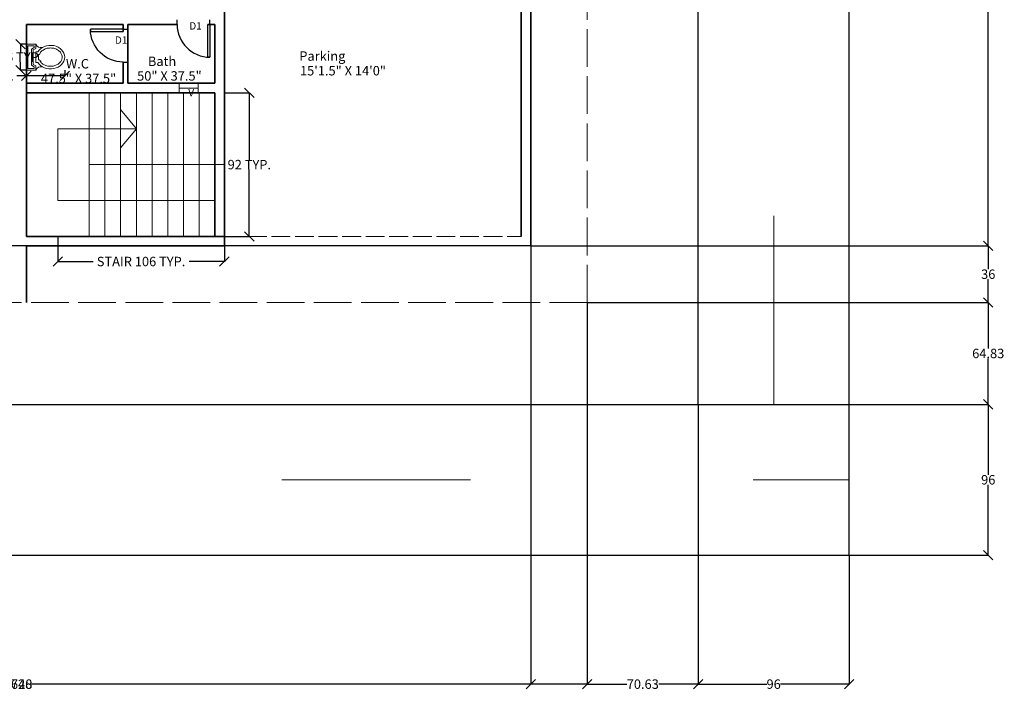
# Model space of a CAD drawing. Units: inches. Extents: x -1198 to -69, y -512 to 437.
# Tile 26 of 50: x -696 to -69, y -512 to -85. Entities that reach past the tile are written whole.
import ezdxf

# ---------------------------------------------------------------- set-up
doc = ezdxf.new("R2010")
doc.units = ezdxf.units.IN
doc.header["$MEASUREMENT"] = 0
doc.linetypes.add('ACAD_ISO02W100', pattern=[15, 12, -3])
doc.linetypes.add('ACAD_ISO03W100', pattern=[30, 12, -18])
for name, color, linetype, lineweight in [('A-ANNO-DIMS', 2, 'Continuous', 18), ('A-ANNO-SYMB', 7, 'Continuous', 18), ('A-AREA-IDEN', 7, 'Continuous', 18), ('A-FLOR-FIXT', 60, 'Continuous', 18), ('A-FLOR-OPEN', 7, 'ACAD_ISO02W100', 18), ('A-FLOR-STRS', 7, 'Continuous', 18), ('A-WALL', 7, 'Continuous', 35), ('C-PROP', 141, 'ACAD_ISO02W100', 18), ('C-ROAD', 7, 'Continuous', 25), ('C-ROAD-CNTR', 7, 'ACAD_ISO03W100', 18), ('Doors', 140, 'Continuous', 25), ('windows', 160, 'Continuous', 18)]:
    doc.layers.add(name, color=color, linetype=linetype, lineweight=lineweight)
doc.styles.get("Standard").update_dxf_attribs({"font": 'arial.ttf'})
doc.dimstyles.get("Standard").update_dxf_attribs({"dimtxt": 6, "dimasz": 6, "dimexe": 0.18, "dimexo": 0.0625, "dimgap": 0.09, "dimtad": 0, "dimtih": 1, "dimtoh": 1, "dimdec": 0, "dimzin": 0, "dimdsep": 46, "dimlunit": 4, "dimtxsty": 'Standard', "dimblk": 'OBLIQUE', "dimcen": 0.09, "dimadec": 0, "dimazin": 0, "dimtfac": 1, "dimtdec": 0, "dimtofl": 0, "dimtmove": 0, "dimatfit": 3, "dimfxl": 1, "dimtolj": 1, "dimtzin": 0, "dimarcsym": 0})

# ---------------------------------------------------------------- blocks, each defined once
blk = doc.blocks.new('A$C7C8779AE')
for p, q in [((0, 0.74), (0, 0.56)), ((0.5, 0.74), (0, 0.74)), ((0.47, 0.71), (0.03, 0.71)), ((0.03, 0.71), (0.03, 0.59)), ((0.03, 0.59), (0.063, 0.59)), ((0.093, 0.64), (0.063, 0.59)), ((0.11, 0.61), (0.08, 0.56)), ((0.093, 0.64), (0.407, 0.64)), ((0.11, 0.61), (0.39, 0.61)), ((0.42, 0.56), (0.39, 0.61)), ((0.437, 0.59), (0.407, 0.64)), ((0.437, 0.59), (0.47, 0.59)), ((0.47, 0.59), (0.47, 0.71)), ((0.5, 0.56), (0.5, 0.74)), ((0, 0.56), (0.08, 0.56)), ((0.15, 0.557), (0.15, 0.52)), ((0.15, 0.557), (0.351, 0.557)), ((0.2, 0.507), (0.2, 0.488)), ((0.2, 0.507), (0.301, 0.507)), ((0.301, 0.507), (0.301, 0.488)), ((0.351, 0.557), (0.351, 0.52)), ((0.42, 0.56), (0.5, 0.56))]:
    blk.add_line(p, q)
for centre, start, end in [((-0.039, 0.461), 344.642, 68.7339), ((0.539, 0.461), 111.2661, 195.358)]:
    blk.add_arc(centre, 0.106, start, end)
blk.add_ellipse((0.251, 0.274), major_axis=(0, 0.274), ratio=0.828948, start_param=0.459479, end_param=5.823706)
blk.add_open_spline([(0.2, 0.488), (0.17, 0.474), (0.164, 0.47), (0.151, 0.46), (0.144, 0.454), (0.13, 0.439), (0.123, 0.431), (0.111, 0.413), (0.106, 0.404), (0.096, 0.384), (0.091, 0.373), (0.084, 0.352), (0.081, 0.34), (0.076, 0.317), (0.075, 0.305), (0.073, 0.282), (0.073, 0.27), (0.074, 0.246), (0.076, 0.234), (0.08, 0.211), (0.083, 0.2), (0.09, 0.178), (0.095, 0.167), (0.104, 0.147), (0.11, 0.138), (0.122, 0.12), (0.128, 0.112), (0.142, 0.097), (0.149, 0.09), (0.165, 0.078), (0.173, 0.073), (0.189, 0.064), (0.197, 0.06), (0.214, 0.055), (0.222, 0.053), (0.239, 0.05), (0.248, 0.05), (0.266, 0.051), (0.276, 0.052), (0.296, 0.057), (0.306, 0.061), (0.325, 0.071), (0.335, 0.077), (0.353, 0.091), (0.361, 0.099), (0.377, 0.117), (0.384, 0.127), (0.398, 0.149), (0.404, 0.161), (0.414, 0.185), (0.418, 0.198), (0.424, 0.225), (0.426, 0.239), (0.428, 0.267), (0.428, 0.281), (0.426, 0.309), (0.424, 0.323), (0.418, 0.349), (0.414, 0.363), (0.404, 0.387), (0.398, 0.399), (0.385, 0.421), (0.378, 0.431), (0.362, 0.449), (0.353, 0.458), (0.338, 0.469), (0.332, 0.474), (0.301, 0.488)], degree=3, knots=[0.459479, 0.459479, 0.459479, 0.459479, 0.567422, 0.567422, 0.720865, 0.720865, 0.874307, 0.874307, 1.02775, 1.02775, 1.181192, 1.181192, 1.334635, 1.334635, 1.488077, 1.488077, 1.64152, 1.64152, 1.794963, 1.794963, 1.948405, 1.948405, 2.101848, 2.101848, 2.25529, 2.25529, 2.408733, 2.408733, 2.562175, 2.562175, 2.715618, 2.715618, 2.86906, 2.86906, 3.022503, 3.022503, 3.175946, 3.175946, 3.356457, 3.356457, 3.536968, 3.536968, 3.717479, 3.717479, 3.89799, 3.89799, 4.078501, 4.078501, 4.259012, 4.259012, 4.439523, 4.439523, 4.620035, 4.620035, 4.800546, 4.800546, 4.981057, 4.981057, 5.161568, 5.161568, 5.342079, 5.342079, 5.52259, 5.52259, 5.703101, 5.703101, 5.823706, 5.823706, 5.823706, 5.823706])
blk = doc.blocks.new('A')
at = {"xscale": 1000, "yscale": 1000, "zscale": 1000}
blk.add_blockref('A$C7C8779AE', (-251, 0), dxfattribs=at)
blk = doc.blocks.new('VENT-12')
at = {"ltscale": 10}
for p, q in [((0, 6), (0, 0)), ((0, 3), (12, 3)), ((12, 6), (12, 0))]:
    blk.add_line(p, q, dxfattribs=at)
blk = doc.blocks.new('DOOR-D1-JAMB3')
for p, q in [((0, 0), (0, -3)), ((20.87, 0), (20.87, -3))]:
    blk.add_line(p, q)
blk.add_lwpolyline([(0, 0), (0, 20.87), (1.3, 20.87), (1.3, 0)], close=True)
blk.add_arc((0, 0), 20.87, 0, 90)
blk = doc.blocks.new('STAIR-RETURN')
at = {"ltscale": 10}
for p, q in [((20, 91.5), (20, 0)), ((30, 91.5), (30, 0)), ((40, 91.5), (40, 0)), ((50, 91.5), (50, 0)), ((60, 91.5), (60, 0)), ((70, 91.5), (70, 0)), ((80, 91.5), (80, 0)), ((90, 91.5), (90, 0)), ((50, 68.62), (40, 80.86)), ((0, 22.87), (0, 68.62)), ((0, 68.62), (50, 68.62)), ((50, 68.62), (40, 56.39)), ((20, 45.75), (106, 45.75)), ((100, 22.87), (0, 22.87))]:
    blk.add_line(p, q, dxfattribs=at)
blk = doc.blocks.new('_Oblique')
at = {"color": 0, "linetype": 'ByBlock', "lineweight": -2}
blk.add_line((-0.5, -0.5), (0.5, 0.5), dxfattribs=at)
blk = doc.blocks.new('*D44')
at = {"layer": 'A-ANNO-DIMS', "color": 0, "lineweight": -2, "ltscale": 10, "transparency": 16777216}
for p, q in [((-691.75, -116.92), (-691.75, -120.7)), ((-667.34, -116.92), (-667.34, -120.7)), ((-691.75, -120.52), (-697.75, -120.52)), ((-667.34, -120.52), (-691.75, -120.52))]:
    blk.add_line(p, q, dxfattribs=at)
at = {"layer": 'DEFPOINTS', "color": 0, "ltscale": 10, "transparency": 16777216}
for p in [(-691.75, -116.86), (-667.34, -116.86), (-691.75, -120.52)]:
    blk.add_point(p, dxfattribs=at)
at = {"layer": 'A-ANNO-DIMS', "color": 0, "lineweight": -2, "ltscale": 10, "transparency": 16777216, "xscale": 6, "yscale": 6, "zscale": 6, "rotation": 180}
blk.add_blockref('_Oblique', (-691.75, -120.52), dxfattribs=at)
at = {"layer": 'A-ANNO-DIMS', "color": 0, "lineweight": -2, "ltscale": 10, "transparency": 16777216, "xscale": 6, "yscale": 6, "zscale": 6}
blk.add_blockref('_Oblique', (-667.34, -120.52), dxfattribs=at)
at = {"layer": 'A-ANNO-DIMS', "color": 0, "ltscale": 10, "transparency": 16777216, "insert": (-720.71, -120.52), "char_height": 6, "attachment_point": 5}
blk.add_mtext('\\A1;WC 24 TYP.', dxfattribs=at)
blk = doc.blocks.new('*D45')
at = {"layer": 'A-ANNO-DIMS', "color": 0, "lineweight": -2, "ltscale": 10, "transparency": 16777216}
for p, q in [((-691.81, -100.37), (-695.59, -100.37)), ((-695.41, -100.37), (-695.41, -105.46)), ((-695.41, -116.86), (-695.41, -111.77)), ((-691.81, -116.86), (-695.59, -116.86))]:
    blk.add_line(p, q, dxfattribs=at)
at = {"layer": 'DEFPOINTS', "color": 0, "ltscale": 10, "transparency": 16777216}
for p in [(-695.41, -100.37), (-691.75, -100.37), (-691.75, -116.86)]:
    blk.add_point(p, dxfattribs=at)
at = {"layer": 'A-ANNO-DIMS', "color": 0, "lineweight": -2, "ltscale": 10, "transparency": 16777216, "xscale": 6, "yscale": 6, "zscale": 6}
for p, rotation in [((-695.41, -100.37), 90), ((-695.41, -116.86), 270)]:
    blk.add_blockref('_Oblique', p, dxfattribs=dict(at, rotation=rotation))
at = {"layer": 'A-ANNO-DIMS', "color": 0, "ltscale": 10, "transparency": 16777216, "insert": (-695.41, -108.61), "char_height": 6, "attachment_point": 5}
blk.add_mtext('\\A1;16 TYP.', dxfattribs=at)
blk = doc.blocks.new('*D54')
at = {"layer": 'A-ANNO-DIMS', "color": 0, "lineweight": -2, "ltscale": 10, "transparency": 16777216}
for p, q in [((-671.75, -222.83), (-671.75, -238.85)), ((-565.75, -222.83), (-565.75, -238.85)), ((-671.75, -238.67), (-649.27, -238.67)), ((-565.75, -238.67), (-588.24, -238.67))]:
    blk.add_line(p, q, dxfattribs=at)
at = {"layer": 'DEFPOINTS', "color": 0, "ltscale": 10, "transparency": 16777216}
for p in [(-671.75, -222.77), (-565.75, -222.77), (-565.75, -238.67)]:
    blk.add_point(p, dxfattribs=at)
at = {"layer": 'A-ANNO-DIMS', "color": 0, "lineweight": -2, "ltscale": 10, "transparency": 16777216, "xscale": 6, "yscale": 6, "zscale": 6, "rotation": 180}
blk.add_blockref('_Oblique', (-671.75, -238.67), dxfattribs=at)
at = {"layer": 'A-ANNO-DIMS', "color": 0, "lineweight": -2, "ltscale": 10, "transparency": 16777216, "xscale": 6, "yscale": 6, "zscale": 6}
blk.add_blockref('_Oblique', (-565.75, -238.67), dxfattribs=at)
at = {"layer": 'A-ANNO-DIMS', "color": 0, "ltscale": 10, "transparency": 16777216, "insert": (-618.75, -238.67), "char_height": 6, "attachment_point": 5}
blk.add_mtext('\\A1;STAIR 106 TYP.', dxfattribs=at)
blk = doc.blocks.new('*D55')
at = {"layer": 'A-ANNO-DIMS', "color": 0, "lineweight": -2, "ltscale": 10, "transparency": 16777216}
for p, q in [((-565.69, -131.27), (-549.67, -131.27)), ((-549.85, -131.27), (-549.85, -173.87)), ((-549.85, -222.77), (-549.85, -180.18)), ((-565.69, -222.77), (-549.67, -222.77))]:
    blk.add_line(p, q, dxfattribs=at)
at = {"layer": 'DEFPOINTS', "color": 0, "ltscale": 10, "transparency": 16777216}
for p in [(-565.75, -131.27), (-549.85, -131.27), (-565.75, -222.77)]:
    blk.add_point(p, dxfattribs=at)
at = {"layer": 'A-ANNO-DIMS', "color": 0, "lineweight": -2, "ltscale": 10, "transparency": 16777216, "xscale": 6, "yscale": 6, "zscale": 6}
for p, rotation in [((-549.85, -131.27), 90), ((-549.85, -222.77), 270)]:
    blk.add_blockref('_Oblique', p, dxfattribs=dict(at, rotation=rotation))
at = {"layer": 'A-ANNO-DIMS', "color": 0, "ltscale": 10, "transparency": 16777216, "insert": (-549.85, -177.02), "char_height": 6, "attachment_point": 5}
blk.add_mtext('\\A1;92 TYP.', dxfattribs=at)
blk = doc.blocks.new('*D60')
at = {"layer": 'A-ANNO-DIMS', "color": 0, "lineweight": -2, "ltscale": 10, "transparency": 16777216}
for p, q in [((-1054.75, -264.83), (-1054.75, -507.84)), ((-334.75, -264.83), (-334.75, -507.84)), ((-1054.75, -507.66), (-701.43, -507.66)), ((-334.75, -507.66), (-688.07, -507.66))]:
    blk.add_line(p, q, dxfattribs=at)
at = {"layer": 'DEFPOINTS', "color": 0, "ltscale": 10, "transparency": 16777216}
for p in [(-1054.75, -264.77), (-334.75, -264.77), (-334.75, -507.66)]:
    blk.add_point(p, dxfattribs=at)
at = {"layer": 'A-ANNO-DIMS', "color": 0, "lineweight": -2, "ltscale": 10, "transparency": 16777216, "xscale": 6, "yscale": 6, "zscale": 6, "rotation": 180}
blk.add_blockref('_Oblique', (-1054.75, -507.66), dxfattribs=at)
at = {"layer": 'A-ANNO-DIMS', "color": 0, "lineweight": -2, "ltscale": 10, "transparency": 16777216, "xscale": 6, "yscale": 6, "zscale": 6}
blk.add_blockref('_Oblique', (-334.75, -507.66), dxfattribs=at)
at = {"layer": 'A-ANNO-DIMS', "color": 0, "ltscale": 10, "transparency": 16777216, "insert": (-694.75, -507.66), "char_height": 6, "attachment_point": 5}
blk.add_mtext('\\A1;720', dxfattribs=at)
blk = doc.blocks.new('*D62')
at = {"layer": 'A-ANNO-DIMS', "color": 0, "lineweight": -2, "ltscale": 10, "transparency": 16777216}
for p, q in [((-1018.75, -228.83), (-1018.75, -507.84)), ((-370.75, -228.83), (-370.75, -507.84)), ((-1018.75, -507.66), (-701.49, -507.66)), ((-370.75, -507.66), (-688.01, -507.66))]:
    blk.add_line(p, q, dxfattribs=at)
at = {"layer": 'DEFPOINTS', "color": 0, "ltscale": 10, "transparency": 16777216}
for p in [(-1018.75, -228.77), (-370.75, -228.77), (-370.75, -507.66)]:
    blk.add_point(p, dxfattribs=at)
at = {"layer": 'A-ANNO-DIMS', "color": 0, "lineweight": -2, "ltscale": 10, "transparency": 16777216, "xscale": 6, "yscale": 6, "zscale": 6, "rotation": 180}
blk.add_blockref('_Oblique', (-1018.75, -507.66), dxfattribs=at)
at = {"layer": 'A-ANNO-DIMS', "color": 0, "lineweight": -2, "ltscale": 10, "transparency": 16777216, "xscale": 6, "yscale": 6, "zscale": 6}
blk.add_blockref('_Oblique', (-370.75, -507.66), dxfattribs=at)
at = {"layer": 'A-ANNO-DIMS', "color": 0, "ltscale": 10, "transparency": 16777216, "insert": (-694.75, -507.66), "char_height": 6, "attachment_point": 5}
blk.add_mtext('\\A1;648', dxfattribs=at)
blk = doc.blocks.new('*D63')
at = {"layer": 'A-ANNO-DIMS', "color": 0, "lineweight": -2, "ltscale": 10, "transparency": 16777216}
for p, q in [((-370.69, 263.23), (-79.37, 263.23)), ((-79.55, 263.23), (-79.55, 20.38)), ((-79.55, -228.77), (-79.55, 14.07)), ((-370.69, -228.77), (-79.37, -228.77))]:
    blk.add_line(p, q, dxfattribs=at)
at = {"layer": 'DEFPOINTS', "color": 0, "ltscale": 10, "transparency": 16777216}
for p in [(-370.75, 263.23), (-79.55, 263.23), (-370.75, -228.77)]:
    blk.add_point(p, dxfattribs=at)
at = {"layer": 'A-ANNO-DIMS', "color": 0, "lineweight": -2, "ltscale": 10, "transparency": 16777216, "xscale": 6, "yscale": 6, "zscale": 6}
for p, rotation in [((-79.55, 263.23), 90), ((-79.55, -228.77), 270)]:
    blk.add_blockref('_Oblique', p, dxfattribs=dict(at, rotation=rotation))
at = {"layer": 'A-ANNO-DIMS', "color": 0, "ltscale": 10, "transparency": 16777216, "insert": (-79.55, 17.23), "char_height": 6, "attachment_point": 5}
blk.add_mtext('\\A1;492', dxfattribs=at)
blk = doc.blocks.new('*D66')
at = {"layer": 'A-ANNO-DIMS', "color": 0, "lineweight": -2, "ltscale": 10, "transparency": 16777216}
for p, q in [((-370.69, -228.77), (-79.37, -228.77)), ((-79.55, -228.77), (-79.55, -243.62)), ((-79.55, -264.77), (-79.55, -249.93)), ((-334.69, -264.77), (-79.37, -264.77))]:
    blk.add_line(p, q, dxfattribs=at)
at = {"layer": 'DEFPOINTS', "color": 0, "ltscale": 10, "transparency": 16777216}
for p in [(-370.75, -228.77), (-79.55, -228.77), (-334.75, -264.77)]:
    blk.add_point(p, dxfattribs=at)
at = {"layer": 'A-ANNO-DIMS', "color": 0, "lineweight": -2, "ltscale": 10, "transparency": 16777216, "xscale": 6, "yscale": 6, "zscale": 6}
for p, rotation in [((-79.55, -228.77), 90), ((-79.55, -264.77), 270)]:
    blk.add_blockref('_Oblique', p, dxfattribs=dict(at, rotation=rotation))
at = {"layer": 'A-ANNO-DIMS', "color": 0, "ltscale": 10, "transparency": 16777216, "insert": (-79.55, -246.77), "char_height": 6, "attachment_point": 5}
blk.add_mtext('\\A1;36', dxfattribs=at)
blk = doc.blocks.new('*D67')
at = {"layer": 'A-ANNO-DIMS', "color": 0, "lineweight": -2, "ltscale": 10, "transparency": 16777216}
for p, q in [((-334.69, -264.77), (-79.37, -264.77)), ((-79.55, -264.77), (-79.55, -294.03)), ((-79.55, -329.6), (-79.55, -300.34)), ((-264.05, -329.6), (-79.37, -329.6))]:
    blk.add_line(p, q, dxfattribs=at)
at = {"layer": 'DEFPOINTS', "color": 0, "ltscale": 10, "transparency": 16777216}
for p in [(-334.75, -264.77), (-264.12, -329.6), (-79.55, -329.6)]:
    blk.add_point(p, dxfattribs=at)
at = {"layer": 'A-ANNO-DIMS', "color": 0, "lineweight": -2, "ltscale": 10, "transparency": 16777216, "xscale": 6, "yscale": 6, "zscale": 6}
for p, rotation in [((-79.55, -264.77), 90), ((-79.55, -329.6), 270)]:
    blk.add_blockref('_Oblique', p, dxfattribs=dict(at, rotation=rotation))
at = {"layer": 'A-ANNO-DIMS', "color": 0, "ltscale": 10, "transparency": 16777216, "insert": (-79.55, -297.19), "char_height": 6, "attachment_point": 5}
blk.add_mtext('\\A1;64.83', dxfattribs=at)
blk = doc.blocks.new('*D68')
at = {"layer": 'A-ANNO-DIMS', "color": 0, "lineweight": -2, "ltscale": 10, "transparency": 16777216}
for p, q in [((-334.75, -264.83), (-334.75, -507.84)), ((-264.12, -329.67), (-264.12, -507.84)), ((-334.75, -507.66), (-309.62, -507.66)), ((-264.12, -507.66), (-289.24, -507.66))]:
    blk.add_line(p, q, dxfattribs=at)
at = {"layer": 'DEFPOINTS', "color": 0, "ltscale": 10, "transparency": 16777216}
for p in [(-334.75, -264.77), (-264.12, -329.6), (-264.12, -507.66)]:
    blk.add_point(p, dxfattribs=at)
at = {"layer": 'A-ANNO-DIMS', "color": 0, "lineweight": -2, "ltscale": 10, "transparency": 16777216, "xscale": 6, "yscale": 6, "zscale": 6, "rotation": 180}
blk.add_blockref('_Oblique', (-334.75, -507.66), dxfattribs=at)
at = {"layer": 'A-ANNO-DIMS', "color": 0, "lineweight": -2, "ltscale": 10, "transparency": 16777216, "xscale": 6, "yscale": 6, "zscale": 6}
blk.add_blockref('_Oblique', (-264.12, -507.66), dxfattribs=at)
at = {"layer": 'A-ANNO-DIMS', "color": 0, "ltscale": 10, "transparency": 16777216, "insert": (-299.43, -507.66), "char_height": 6, "attachment_point": 5}
blk.add_mtext('\\A1;70.63', dxfattribs=at)
blk = doc.blocks.new('*D69')
at = {"layer": 'A-ANNO-DIMS', "color": 0, "lineweight": -2, "ltscale": 10, "transparency": 16777216}
for p, q in [((-264.12, -329.67), (-264.12, -507.84)), ((-168.12, -425.67), (-168.12, -507.84)), ((-264.12, -507.66), (-220.5, -507.66)), ((-168.12, -507.66), (-211.73, -507.66))]:
    blk.add_line(p, q, dxfattribs=at)
at = {"layer": 'DEFPOINTS', "color": 0, "ltscale": 10, "transparency": 16777216}
for p in [(-264.12, -329.6), (-168.12, -425.6), (-168.12, -507.66)]:
    blk.add_point(p, dxfattribs=at)
at = {"layer": 'A-ANNO-DIMS', "color": 0, "lineweight": -2, "ltscale": 10, "transparency": 16777216, "xscale": 6, "yscale": 6, "zscale": 6, "rotation": 180}
blk.add_blockref('_Oblique', (-264.12, -507.66), dxfattribs=at)
at = {"layer": 'A-ANNO-DIMS', "color": 0, "lineweight": -2, "ltscale": 10, "transparency": 16777216, "xscale": 6, "yscale": 6, "zscale": 6}
blk.add_blockref('_Oblique', (-168.12, -507.66), dxfattribs=at)
at = {"layer": 'A-ANNO-DIMS', "color": 0, "ltscale": 10, "transparency": 16777216, "insert": (-216.12, -507.66), "char_height": 6, "attachment_point": 5}
blk.add_mtext('\\A1;96', dxfattribs=at)
blk = doc.blocks.new('*D70')
at = {"layer": 'A-ANNO-DIMS', "color": 0, "lineweight": -2, "ltscale": 10, "transparency": 16777216}
for p, q in [((-264.05, -329.6), (-79.37, -329.6)), ((-79.55, -329.6), (-79.55, -374.45)), ((-79.55, -425.6), (-79.55, -380.76)), ((-168.05, -425.6), (-79.37, -425.6))]:
    blk.add_line(p, q, dxfattribs=at)
at = {"layer": 'DEFPOINTS', "color": 0, "ltscale": 10, "transparency": 16777216}
for p in [(-264.12, -329.6), (-168.12, -425.6), (-79.55, -425.6)]:
    blk.add_point(p, dxfattribs=at)
at = {"layer": 'A-ANNO-DIMS', "color": 0, "lineweight": -2, "ltscale": 10, "transparency": 16777216, "xscale": 6, "yscale": 6, "zscale": 6}
for p, rotation in [((-79.55, -329.6), 90), ((-79.55, -425.6), 270)]:
    blk.add_blockref('_Oblique', p, dxfattribs=dict(at, rotation=rotation))
at = {"layer": 'A-ANNO-DIMS', "color": 0, "ltscale": 10, "transparency": 16777216, "insert": (-79.55, -377.6), "char_height": 6, "attachment_point": 5}
blk.add_mtext('\\A1;96', dxfattribs=at)
blk = doc.blocks.new('*D75')
at = {"layer": 'A-ANNO-DIMS', "color": 0, "lineweight": -2, "ltscale": 10, "transparency": 16777216}
for p, q in [((-376.81, -44.27), (-1188.2, -44.27)), ((-1188.02, -44.27), (-1188.02, -133.37)), ((-1188.02, -228.77), (-1188.02, -139.68)), ((-370.81, -228.77), (-1188.2, -228.77))]:
    blk.add_line(p, q, dxfattribs=at)
at = {"layer": 'DEFPOINTS', "color": 0, "ltscale": 10, "transparency": 16777216}
for p in [(-1188.02, -44.27), (-376.75, -44.27), (-370.75, -228.77)]:
    blk.add_point(p, dxfattribs=at)
at = {"layer": 'A-ANNO-DIMS', "color": 0, "lineweight": -2, "ltscale": 10, "transparency": 16777216, "xscale": 6, "yscale": 6, "zscale": 6}
for p, rotation in [((-1188.02, -44.27), 90), ((-1188.02, -228.77), 270)]:
    blk.add_blockref('_Oblique', p, dxfattribs=dict(at, rotation=rotation))
at = {"layer": 'A-ANNO-DIMS', "color": 0, "ltscale": 10, "transparency": 16777216, "insert": (-1188.02, -136.52), "char_height": 6, "attachment_point": 5}
blk.add_mtext('\\A1;184.5', dxfattribs=at)

msp = doc.modelspace()

# ---------------------------------------------------------------- linework, layer by layer
at = {"layer": 'A-FLOR-OPEN'}
for p, q in [((-565.7509, -222.7723), (-376.7509, -222.7723)), ((-691.7509, -228.7723), (-370.7509, -228.7723))]:
    msp.add_line(p, q, dxfattribs=at)
at = {"layer": 'A-WALL', "ltscale": 10}
for p, q in [((-370.7509, -228.7723), (-370.7509, 263.2277)), ((-376.7509, -222.7723), (-376.7509, 257.2277)), ((-565.7509, -44.2723), (-565.7509, -125.2723)), ((-641.2509, -87.7723), (-691.7509, -87.7723)), ((-691.7509, -87.7723), (-691.7509, -125.2723)), ((-691.7509, -87.7723), (-691.7509, -222.7723)), ((-630.0669, -87.7723), (-641.2509, -87.7723)), ((-630.0669, -87.7723), (-630.0669, -92.2048)), ((-595.782, -87.7723), (-627.0669, -87.7723)), ((-627.0669, -87.7723), (-627.0669, -125.2723)), ((-571.7509, -87.7723), (-576.2167, -87.7723)), ((-571.7509, -87.7723), (-571.7509, -125.2723)), ((-565.7509, -87.7723), (-565.7509, -131.2723)), ((-630.0669, -111.7701), (-630.0669, -125.2723)), ((-641.2509, -125.2723), (-691.7509, -125.2723)), ((-630.0669, -125.2723), (-641.2509, -125.2723)), ((-571.7509, -125.2723), (-627.0669, -125.2723)), ((-571.7509, -131.2723), (-691.7509, -131.2723)), ((-691.7509, -131.2723), (-691.7509, -222.7723)), ((-571.7509, -131.2723), (-571.7509, -222.7723)), ((-565.7509, -131.2723), (-565.7509, -228.7723)), ((-691.7509, -222.7723), (-565.7509, -222.7723)), ((-691.7509, -222.7723), (-565.7509, -222.7723)), ((-691.7509, -228.7723), (-691.7509, -264.7723)), ((-691.7509, -228.7723), (-565.7509, -228.7723)), ((-691.7509, -228.7723), (-565.7509, -228.7723))]:
    msp.add_line(p, q, dxfattribs=at)
at = {"layer": 'C-PROP', "ltscale": 2}
msp.add_lwpolyline([(-1054.7509, 299.2277), (-334.7509, 299.2277), (-334.7509, -264.7723), (-1054.7509, -264.7723)], close=True, dxfattribs=at)
at = {"layer": 'C-ROAD', "ltscale": 10}
for p, q in [((-264.1167, -329.6039), (-264.1167, 374.1612)), ((-168.1167, -425.6039), (-168.1167, 374.1612)), ((-1129.1823, -329.6039), (-264.1167, -329.6039)), ((-1129.1823, -425.6039), (-168.1167, -425.6039))]:
    msp.add_line(p, q, dxfattribs=at)
at = {"layer": 'C-ROAD-CNTR', "ltscale": 10}
for p, q in [((-216.1167, -329.6039), (-216.1167, 374.1612)), ((-1129.1823, -377.6039), (-168.1167, -377.6039))]:
    msp.add_line(p, q, dxfattribs=at)

# ---------------------------------------------------------------- block references
at = {"layer": 'A-FLOR-FIXT', "ltscale": 10, "xscale": 0.0329718540314781, "yscale": 0.0329718540314781, "zscale": 0.0329718540314781, "rotation": 89.99999999999999}
msp.add_blockref('A', (-667.3364, -108.5941), dxfattribs=at)
at = {"layer": 'A-FLOR-STRS'}
msp.add_blockref('STAIR-RETURN', (-671.751, -222.772), dxfattribs=at)
at = {"layer": 'Doors', "rotation": 180}
msp.add_blockref('DOOR-D1-JAMB3', (-574.9123, -87.7723), dxfattribs=at)
at = {"layer": 'Doors', "extrusion": (0, 0, -1), "zscale": -1, "rotation": 269.9999999999994}
msp.add_blockref('DOOR-D1-JAMB3', (630.0669, -90.9004), dxfattribs=at)
at = {"layer": 'windows', "rotation": 180}
msp.add_blockref('VENT-12', (-582.4789, -125.2727), dxfattribs=at)

# ---------------------------------------------------------------- texts
at = {"layer": 'A-ANNO-SYMB', "ltscale": 10}
for s, height, p in [('D1', 4.69957, (-588.0676, -91.05)), ('D1', 4.69957, (-635.4254, -100.0945)), ('V', 4.6996, (-588.6937, -133.6031))]:
    msp.add_text(s, height=height, dxfattribs=at).set_placement(p)
at = {"layer": 'A-AREA-IDEN', "ltscale": 10, "char_height": 6, "attachment_point": 1}
for s, insert in [('Parking', (-518.0415, -104.9183)), ('W.C', (-666.5723, -109.8143)), ('Bath', (-614.407, -108.2495)), ('47.5" X 37.5"', (-682.5231, -119.1414)), ('50" X 37.5"', (-621.2707, -117.5766)), ('15\'1.5" X 14\'0"', (-517.6221, -114.2454))]:
    msp.add_mtext_dynamic_manual_height_columns(s, width=57.976527, gutter_width=30, heights=[0], dxfattribs=dict(at, insert=insert))

# ---------------------------------------------------------------- dimensions: what is measured, and where the dimension line sits
at = {"layer": 'A-ANNO-DIMS', "ltscale": 10}
for base, p1, p2, override, picture, middle in [((-79.5507, 263.2277), (-370.7509, -228.7723), (-370.7509, 263.2277), {"dimdec": 0, "dimlfac": 1, "dimrnd": 0, "dimzin": 0, "dimdsep": 46, "dimlunit": 2}, '*D63', (-79.5507, 17.2277)), ((-1188.0248, -44.2723), (-370.7509, -228.7723), (-376.7509, -44.2723), {"dimdec": 1, "dimlfac": 1, "dimrnd": 0, "dimzin": 0, "dimdsep": 46, "dimlunit": 2}, '*D75', (-1188.0248, -136.5223)), ((-79.5507, -228.7723), (-334.7509, -264.7723), (-370.7509, -228.7723), {"dimdec": 0, "dimlfac": 1, "dimrnd": 0, "dimzin": 0, "dimdsep": 46, "dimlunit": 2}, '*D66', (-79.5507, -246.7723)), ((-79.5507, -329.6039), (-334.7509, -264.7723), (-264.1167, -329.6039), {"dimdec": 2, "dimlfac": 1, "dimrnd": 0, "dimzin": 0, "dimdsep": 46, "dimlunit": 2}, '*D67', (-79.5507, -297.1881)), ((-79.5507, -425.6039), (-264.1167, -329.6039), (-168.1167, -425.6039), {"dimdec": 0, "dimlfac": 1, "dimrnd": 0, "dimzin": 0, "dimdsep": 46, "dimlunit": 2}, '*D70', (-79.5507, -377.6039))]:
    dim = msp.add_linear_dim(base=base, p1=p1, p2=p2, angle=90, dimstyle='Standard', override=override, dxfattribs=at)
    dim.commit()
    dim.dimension.update_dxf_attribs({"geometry": picture, "text_midpoint": middle})
for base, p1, p2, angle, text, picture, middle in [((-695.413, -100.3697), (-691.7509, -116.8556), (-691.7509, -100.3697), 90, '<> TYP.', '*D45', (-695.413, -108.6126)), ((-691.7509, -120.5177), (-667.3364, -116.8556), (-691.7509, -116.8556), 180, 'WC <> TYP.', '*D44', (-720.7133, -120.5177)), ((-549.8508694019, -131.2723442916), (-565.7508694019, -222.7723442916), (-565.7508694019, -131.2723442916), 90, '<> TYP.', '*D55', (-549.8508694019, -177.0223442916))]:
    dim = msp.add_linear_dim(base=base, p1=p1, p2=p2, angle=angle, text=text, dimstyle='Standard', override={"dimdec": 0, "dimlfac": 1, "dimrnd": 0, "dimzin": 0, "dimdsep": 46, "dimlunit": 2}, dxfattribs=at)
    dim.commit()
    dim.dimension.update_dxf_attribs({"geometry": picture, "text_midpoint": middle})
dim = msp.add_linear_dim(base=(-565.7509, -238.6723), p1=(-671.7509, -222.7723), p2=(-565.7509, -222.7723), text='STAIR <> TYP.', dimstyle='Standard', override={"dimdec": 0, "dimlfac": 1, "dimrnd": 0, "dimzin": 0, "dimdsep": 46, "dimlunit": 2}, dxfattribs=at)
dim.commit()
dim.dimension.update_dxf_attribs({"geometry": '*D54', "text_midpoint": (-618.7509, -238.6723)})
for base, p1, p2, override, picture, middle in [((-370.7509, -507.6552), (-1018.7509, -228.7723), (-370.7509, -228.7723), {"dimdec": 0, "dimlfac": 1, "dimrnd": 0, "dimzin": 0, "dimdsep": 46, "dimlunit": 2}, '*D62', (-694.7509, -507.6552)), ((-334.7509, -507.6552), (-1054.7509, -264.7723), (-334.7509, -264.7723), {"dimdec": 0, "dimlfac": 1, "dimrnd": 0, "dimzin": 0, "dimdsep": 46, "dimlunit": 2}, '*D60', (-694.7509, -507.6552)), ((-264.1167, -507.6552), (-334.7509, -264.7723), (-264.1167, -329.6039), {"dimdec": 2, "dimlfac": 1, "dimrnd": 0, "dimzin": 0, "dimdsep": 46, "dimlunit": 2}, '*D68', (-299.4338, -507.6552)), ((-168.1167, -507.6552), (-264.1167, -329.6039), (-168.1167, -425.6039), {"dimdec": 0, "dimlfac": 1, "dimrnd": 0, "dimzin": 0, "dimdsep": 46, "dimlunit": 2}, '*D69', (-216.1167, -507.6552))]:
    dim = msp.add_linear_dim(base=base, p1=p1, p2=p2, dimstyle='Standard', override=override, dxfattribs=at)
    dim.commit()
    dim.dimension.update_dxf_attribs({"geometry": picture, "text_midpoint": middle})

doc.saveas('drawing.dxf')
